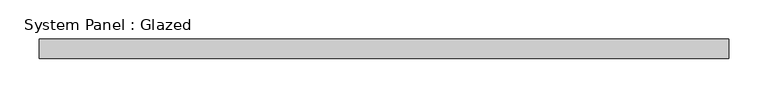
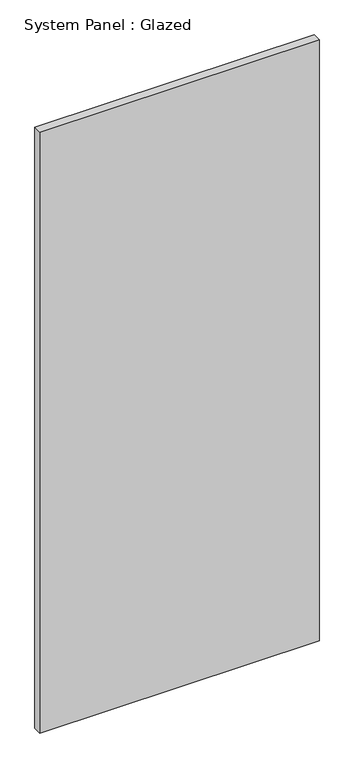
"""IFC4 building model written with IfcOpenShell, lengths in millimetres: plate geometry, System Panel : Glazed."""

from ifc_helpers import new_model, si_unit, origin, origin_with_axes, place, context, project, spatial, polyline, outline, extrude, source, transform, mapped, element, save


def system_panel_glazed_3ab3cb8c(model_context):
    return source(origin(), model_context, "Body", "SweptSolid", [
        extrude(outline(polyline([(441.325, 19.05), (-441.325, 19.05), (-441.325, 44.45), (441.325, 44.45), (441.325, 19.05)])), origin_with_axes(), (0.0, 0.0, 1.0), 2006.6),
    ])


if __name__ == "__main__":
    model = new_model("IFC4")
    model_context = context("Model", 3, world=origin())
    ifc_project = project(units=[si_unit("LENGTHUNIT", "METRE", prefix="MILLI")], contexts=[model_context])
    site = spatial("IfcSite", under=ifc_project)
    building = spatial("IfcBuilding", under=site)
    placement = place(None, origin())
    system_panel_glazed_shape = system_panel_glazed_3ab3cb8c(model_context)
    element("IfcPlate", 1, ObjectType="System Panel : Glazed", at=placement, inside=building, context=model_context, shape_type="MappedRepresentation", body=[
        mapped(system_panel_glazed_shape, transform((0.0, 0.0, 0.0), x_axis=(1.0, 0.0, 0.0), y_axis=(0.0, 1.0, 0.0), z_axis=(0.0, 0.0, 1.0))),
    ])
    save(model, "model.ifc")

# Revit data of these elements
# Type "System Panel : Glazed"
#   Construction Type Id = "GSP4R"
#   Analytic Construction = "1/8 in Pilkington single glazing"
#   Visual Light Transmittance = 0.9
#   Solar Heat Gain Coefficient = 0.86
#   Heat Transfer Coefficient (U) = 1.18115 BTU/(h·ft²·°F)
#   Define Thermal Properties by = 1
# Element 1 (IfcPlate, "System Panel : Glazed")
#   Materials on its faces: "Glass"
# Materials
#   "Glass": class "Glass", colour RGB 0 128 192, transparency 0.75, Description = "Soda Lime Glass", Cost = 0
